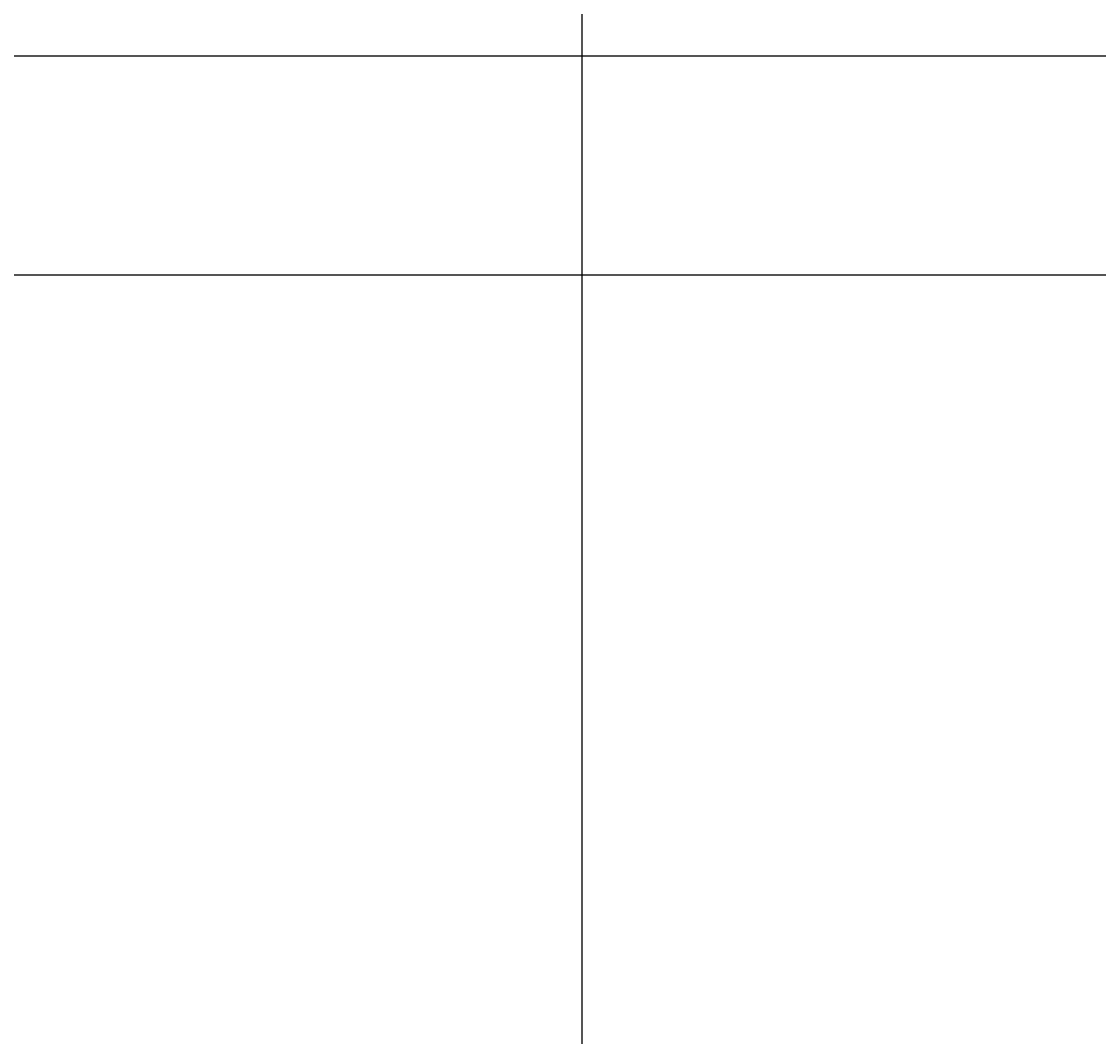
# Model space of a CAD drawing. Units: inches. Extents: x 35362 to 73946, y 43607 to 67532.
# Tile 74 of 134: x 49711 to 50119, y 46919 to 47304. Entities that reach past the tile are written whole.
import ezdxf

# ---------------------------------------------------------------- set-up
doc = ezdxf.new("R2010")
doc.units = ezdxf.units.IN
doc.header["$MEASUREMENT"] = 0
doc.layers.add('A-ANNO-DIMS', color=2, linetype='Continuous', lineweight=18)
doc.styles.get("Standard").update_dxf_attribs({"font": 'arial.ttf'})
doc.dimstyles.get("Standard").update_dxf_attribs({"dimtxt": 0.18, "dimasz": 0.18, "dimexe": 0.18, "dimexo": 0.0625, "dimgap": 0.09, "dimtad": 0, "dimtih": 1, "dimtoh": 1, "dimdec": 4, "dimzin": 0, "dimdsep": 46, "dimtxsty": 'Standard', "dimcen": 0.09, "dimadec": 0, "dimazin": 0, "dimtfac": 1, "dimtdec": 4, "dimtofl": 0, "dimtmove": 0, "dimatfit": 3, "dimfxl": 1, "dimtolj": 1, "dimtzin": 0, "dimarcsym": 0})

# ---------------------------------------------------------------- blocks, each defined once
blk = doc.blocks.new('*D11')
at = {"layer": 'A-ANNO-DIMS', "color": 0, "lineweight": -2, "transparency": 16777216}
for p, q in [((47978.66, 56028.77), (47978.66, 43606.68)), ((53109.76, 56028.77), (53109.76, 43606.68)), ((47978.84, 43606.86), (50543.87, 43606.86)), ((53109.58, 43606.86), (50544.55, 43606.86))]:
    blk.add_line(p, q, dxfattribs=at)
at = {"layer": 'A-ANNO-DIMS', "color": 0, "transparency": 16777216}
for points in [[(47978.84, 43606.89), (47978.84, 43606.83), (47978.66, 43606.86)], [(53109.58, 43606.89), (53109.58, 43606.83), (53109.76, 43606.86)]]:
    blk.add_solid(points, dxfattribs=at)
at = {"layer": 'Defpoints', "color": 0, "transparency": 16777216}
for p in [(47978.66, 56028.84), (53109.76, 56028.84), (53109.76, 43606.86)]:
    blk.add_point(p, dxfattribs=at)
at = {"layer": 'A-ANNO-DIMS', "color": 0, "transparency": 16777216, "insert": (50544.21, 43606.86), "char_height": 0.18, "attachment_point": 5}
blk.add_mtext('\\A1;5131', dxfattribs=at)
blk = doc.blocks.new('*D13')
at = {"layer": 'A-ANNO-DIMS', "color": 0, "lineweight": -2, "transparency": 16777216}
for p, q in [((48373.49, 51694.02), (48373.49, 43606.68)), ((51029.04, 51694.02), (51029.04, 43606.68)), ((48373.67, 43606.86), (49700.8, 43606.86)), ((51028.86, 43606.86), (49701.73, 43606.86))]:
    blk.add_line(p, q, dxfattribs=at)
at = {"layer": 'A-ANNO-DIMS', "color": 0, "transparency": 16777216}
for points in [[(48373.67, 43606.89), (48373.67, 43606.83), (48373.49, 43606.86)], [(51028.86, 43606.89), (51028.86, 43606.83), (51029.04, 43606.86)]]:
    blk.add_solid(points, dxfattribs=at)
at = {"layer": 'Defpoints', "color": 0, "transparency": 16777216}
for p in [(48373.49, 51694.09), (51029.04, 51694.09), (51029.04, 43606.86)]:
    blk.add_point(p, dxfattribs=at)
at = {"layer": 'A-ANNO-DIMS', "color": 0, "transparency": 16777216, "insert": (49701.27, 43606.86), "char_height": 0.18, "attachment_point": 5}
blk.add_mtext('\\A1;2655.6', dxfattribs=at)
blk = doc.blocks.new('*D17')
at = {"layer": 'A-ANNO-DIMS', "color": 0, "lineweight": -2, "transparency": 16777216}
for p, q in [((49923.31, 61293.22), (49923.31, 43606.68)), ((51913.93, 61293.22), (51913.93, 43606.68)), ((49923.49, 43606.86), (50918.16, 43606.86)), ((51913.75, 43606.86), (50919.07, 43606.86))]:
    blk.add_line(p, q, dxfattribs=at)
at = {"layer": 'A-ANNO-DIMS', "color": 0, "transparency": 16777216}
for points in [[(49923.49, 43606.89), (49923.49, 43606.83), (49923.31, 43606.86)], [(51913.75, 43606.89), (51913.75, 43606.83), (51913.93, 43606.86)]]:
    blk.add_solid(points, dxfattribs=at)
at = {"layer": 'Defpoints', "color": 0, "transparency": 16777216}
for p in [(49923.31, 61293.29), (51913.93, 61293.29), (51913.93, 43606.86)]:
    blk.add_point(p, dxfattribs=at)
at = {"layer": 'A-ANNO-DIMS', "color": 0, "transparency": 16777216, "insert": (50918.62, 43606.86), "char_height": 0.18, "attachment_point": 5}
blk.add_mtext('\\A1;1990.6', dxfattribs=at)
blk = doc.blocks.new('*D43')
at = {"layer": 'A-ANNO-DIMS', "color": 0, "lineweight": -2, "transparency": 16777216}
for p, q in [((62004.67, 47625.18), (35361.77, 47625.18)), ((35361.95, 47625), (35361.95, 47416.9)), ((35361.95, 47208.43), (35361.95, 47416.53)), ((62004.67, 47208.25), (35361.77, 47208.25))]:
    blk.add_line(p, q, dxfattribs=at)
at = {"layer": 'A-ANNO-DIMS', "color": 0, "transparency": 16777216}
for points in [[(35361.92, 47625), (35361.98, 47625), (35361.95, 47625.18)], [(35361.92, 47208.43), (35361.98, 47208.43), (35361.95, 47208.25)]]:
    blk.add_solid(points, dxfattribs=at)
at = {"layer": 'Defpoints', "color": 0, "transparency": 16777216}
for p in [(62004.73, 47625.18), (35361.95, 47208.25), (62004.73, 47208.25)]:
    blk.add_point(p, dxfattribs=at)
at = {"layer": 'A-ANNO-DIMS', "color": 0, "transparency": 16777216, "insert": (35361.95, 47416.72), "char_height": 0.18, "attachment_point": 5}
blk.add_mtext('\\A1;416.9', dxfattribs=at)
blk = doc.blocks.new('*D67')
at = {"layer": 'A-ANNO-DIMS', "color": 0, "lineweight": -2, "transparency": 16777216}
for p, q in [((56873.54, 53351.53), (35361.77, 53351.53)), ((35361.95, 53351.35), (35361.95, 49400.89)), ((35361.95, 45450.07), (35361.95, 49400.53)), ((53793.58, 45449.89), (35361.77, 45449.89))]:
    blk.add_line(p, q, dxfattribs=at)
at = {"layer": 'A-ANNO-DIMS', "color": 0, "transparency": 16777216}
for points in [[(35361.92, 53351.35), (35361.98, 53351.35), (35361.95, 53351.53)], [(35361.92, 45450.07), (35361.98, 45450.07), (35361.95, 45449.89)]]:
    blk.add_solid(points, dxfattribs=at)
at = {"layer": 'Defpoints', "color": 0, "transparency": 16777216}
for p in [(35361.95, 53351.53), (56873.6, 53351.53), (53793.64, 45449.89)]:
    blk.add_point(p, dxfattribs=at)
at = {"layer": 'A-ANNO-DIMS', "color": 0, "transparency": 16777216, "insert": (35361.95, 49400.71), "char_height": 0.18, "attachment_point": 5}
blk.add_mtext('\\A1;7901.6', dxfattribs=at)
blk = doc.blocks.new('*D90')
at = {"layer": 'A-ANNO-DIMS', "color": 0, "lineweight": -2, "transparency": 16777216}
for p, q in [((53707.72, 47291.29), (35361.77, 47291.29)), ((35361.95, 47291.11), (35361.95, 46710.26)), ((35361.95, 46129.06), (35361.95, 46709.9)), ((53793.58, 46128.88), (35361.77, 46128.88))]:
    blk.add_line(p, q, dxfattribs=at)
at = {"layer": 'A-ANNO-DIMS', "color": 0, "transparency": 16777216}
for points in [[(35361.92, 47291.11), (35361.98, 47291.11), (35361.95, 47291.29)], [(35361.92, 46129.06), (35361.98, 46129.06), (35361.95, 46128.88)]]:
    blk.add_solid(points, dxfattribs=at)
at = {"layer": 'Defpoints', "color": 0, "transparency": 16777216}
for p in [(53707.78, 47291.29), (35361.95, 46128.88), (53793.64, 46128.88)]:
    blk.add_point(p, dxfattribs=at)
at = {"layer": 'A-ANNO-DIMS', "color": 0, "transparency": 16777216, "insert": (35361.95, 46710.08), "char_height": 0.18, "attachment_point": 5}
blk.add_mtext('\\A1;1162.4', dxfattribs=at)

msp = doc.modelspace()

# ---------------------------------------------------------------- dimensions: what is measured, and where the dimension line sits
at = {"layer": 'A-ANNO-DIMS'}
for base, p1, p2, override, picture, middle in [((51913.931, 43606.859), (49923.307, 61293.286), (51913.931, 61293.286), {"dimdec": 1, "dimlfac": 1, "dimrnd": 0, "dimzin": 0, "dimdsep": 46, "dimlunit": 2}, '*D17', (50918.619, 43606.859)), ((53109.76, 43606.859), (47978.665, 56028.836), (53109.76, 56028.836), {"dimdec": 0, "dimlfac": 1, "dimrnd": 0, "dimzin": 0, "dimdsep": 46, "dimlunit": 2}, '*D11', (50544.212, 43606.859)), ((51029.043, 43606.859), (48373.492, 51694.087), (51029.043, 51694.087), {"dimdec": 1, "dimlfac": 1, "dimrnd": 0, "dimzin": 0, "dimdsep": 46, "dimlunit": 2}, '*D13', (49701.267, 43606.859))]:
    dim = msp.add_linear_dim(base=base, p1=p1, p2=p2, dimstyle='Standard', override=override, dxfattribs=at)
    dim.commit()
    dim.dimension.update_dxf_attribs({"geometry": picture, "text_midpoint": middle})
for base, p1, p2, picture, middle in [((35361.949, 53351.529), (53793.638, 45449.894), (56873.602, 53351.529), '*D67', (35361.949, 49400.712)), ((35361.949, 47208.25), (62004.728, 47625.181), (62004.728, 47208.25), '*D43', (35361.949, 47416.715)), ((35361.949, 46128.878), (53707.781, 47291.285), (53793.638, 46128.878), '*D90', (35361.949, 46710.081))]:
    dim = msp.add_linear_dim(base=base, p1=p1, p2=p2, angle=90, dimstyle='Standard', override={"dimdec": 1, "dimlfac": 1, "dimrnd": 0, "dimzin": 0, "dimdsep": 46, "dimlunit": 2}, dxfattribs=at)
    dim.commit()
    dim.dimension.update_dxf_attribs({"geometry": picture, "text_midpoint": middle})

doc.saveas('drawing.dxf')
